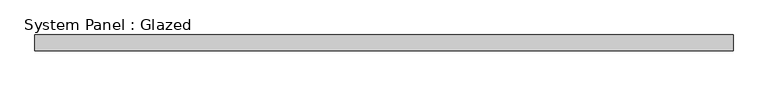
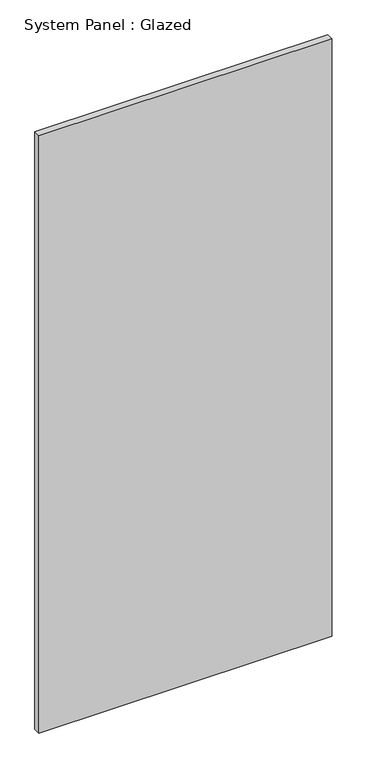
"""IFC4 building model written with IfcOpenShell, lengths in millimetres: plate geometry, System Panel : Glazed."""

from ifc_helpers import new_model, si_unit, origin, origin_with_axes, place, context, project, spatial, polyline, outline, extrude, source, transform, mapped, element, save


def system_panel_glazed_7d86dfa2(model_context):
    return source(origin(), model_context, "Body", "SweptSolid", [
        extrude(outline(polyline([(556.814808, 24.5), (-556.814808, 24.5), (-556.814808, 49.5), (556.814808, 49.5), (556.814808, 24.5)])), origin_with_axes(), (0.0, 0.0, 1.0), 2400.0),
    ])


if __name__ == "__main__":
    model = new_model("IFC4")
    model_context = context("Model", 3, world=origin())
    ifc_project = project(units=[si_unit("LENGTHUNIT", "METRE", prefix="MILLI")], contexts=[model_context])
    site = spatial("IfcSite", under=ifc_project)
    building = spatial("IfcBuilding", under=site)
    placement = place(None, origin())
    system_panel_glazed_shape = system_panel_glazed_7d86dfa2(model_context)
    element("IfcPlate", 1, ObjectType="System Panel : Glazed", at=placement, inside=building, context=model_context, shape_type="MappedRepresentation", body=[
        mapped(system_panel_glazed_shape, transform((0.0, 0.0, 0.0), x_axis=(1.0, 0.0, 0.0), y_axis=(0.0, 1.0, 0.0), z_axis=(0.0, 0.0, 1.0))),
    ])
    save(model, "model.ifc")

# Revit data of these elements
# Type "System Panel : Glazed"
#   Keynote = "H11"
#   Construction Type Id = "GSP4R"
#   Analytic Construction = "1/8 in Pilkington single glazing"
#   Visual Light Transmittance = 0.9
#   Solar Heat Gain Coefficient = 0.86
#   Heat Transfer Coefficient (U) = 6.7069 W/(m²·K)
#   Define Thermal Properties by = 1
# Element 1 (IfcPlate, "System Panel : Glazed")
#   Materials on its faces: "Glass"
# Materials
#   "Glass": class "Glass", colour RGB 0 128 192, transparency 0.9, Description = "Soda Lime Glass", Cost = 0
